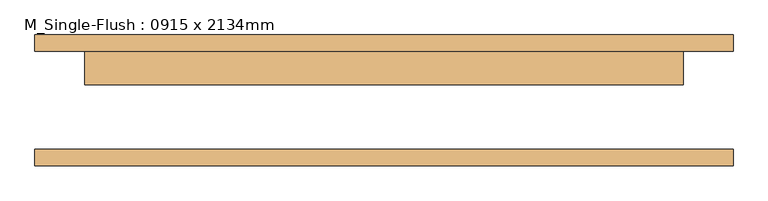
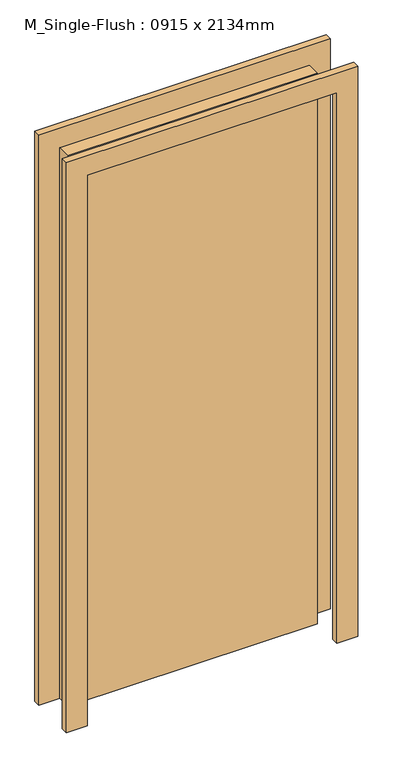
"""IFC4 building model written with IfcOpenShell, lengths in millimetres: door geometry, M_Single-Flush : 0915 x 2134mm."""

from ifc_helpers import new_model, si_unit, frame, origin, origin_with_axes, place, context, project, spatial, polyline, outline, extrude, source, transform, mapped, element, save


def m_single_flush_0915_x_2134mm_138fd904(model_context):
    return source(origin(), model_context, "Body", "SweptSolid", [
        extrude(outline(polyline([(2210.0, -533.5), (0.0, -533.5), (0.0, -457.5), (2134.0, -457.5), (2134.0, 457.5), (0.0, 457.5), (0.0, 533.5), (2210.0, 533.5), (2210.0, -533.5)])), frame((0.0, 75.0, 0.0), z_axis=(0.0, 1.0, 0.0), x_axis=(0.0, 0.0, 1.0)), (0.0, 0.0, 1.0), 25.0),
        extrude(outline(polyline([(2210.0, 533.5), (2210.0, -533.5), (0.0, -533.5), (0.0, -457.5), (2134.0, -457.5), (2134.0, 457.5), (0.0, 457.5), (0.0, 533.5), (2210.0, 533.5)])), frame((0.0, -100.0, 0.0), z_axis=(0.0, 1.0, 0.0), x_axis=(0.0, 0.0, 1.0)), (0.0, 0.0, 1.0), 25.0),
        extrude(outline(polyline([(457.5, 24.0), (-457.5, 24.0), (-457.5, 75.0), (457.5, 75.0), (457.5, 24.0)])), origin_with_axes(), (0.0, 0.0, 1.0), 2134.0),
    ])


if __name__ == "__main__":
    model = new_model("IFC4")
    model_context = context("Model", 3, world=origin())
    ifc_project = project(units=[si_unit("LENGTHUNIT", "METRE", prefix="MILLI")], contexts=[model_context])
    site = spatial("IfcSite", under=ifc_project)
    building = spatial("IfcBuilding", under=site)
    placement = place(None, origin())
    m_single_flush_0915_x_2134mm_shape = m_single_flush_0915_x_2134mm_138fd904(model_context)
    element("IfcDoor", 1, ObjectType="M_Single-Flush : 0915 x 2134mm", at=placement, inside=building, context=model_context, shape_type="MappedRepresentation", body=[
        mapped(m_single_flush_0915_x_2134mm_shape, transform((0.0, 0.0, 0.0), x_axis=(1.0, 0.0, 0.0), y_axis=(0.0, 1.0, 0.0), z_axis=(0.0, 0.0, 1.0))),
    ])
    save(model, "model.ifc")

# Revit data of these elements
# Type "M_Single-Flush : 0915 x 2134mm"
#   Type Mark = "20"
#   Construction Type Id = "MDOOR"
#   Analytic Construction = "Metal"
#   Thickness = 0.051 m
#   Thermal Resistance (R) = 0.270117 (m²·K)/W
#   Heat Transfer Coefficient (U) = 3.7021 W/(m²·K)
#   Height = 2.134 m
#   Trim Projection Ext = 0.025 m
#   Trim Projection Int = 0.025 m
#   Trim Width = 0.076 m
#   Width = 0.915 m
#   Define Thermal Properties by = 1
#   Define Thermal Properties by = 1
#   Door Material = Door - Panel
#   Frame Material = Door - Frame
#   Visual Light Transmittance = 0
#   Solar Heat Gain Coefficient = 0
#   Function = (empty or 0)
#   Wall Closure = (empty or 0)
# Element 1 (IfcDoor, "M_Single-Flush : 0915 x 2134mm")
#   Materials on its faces: "Door - Frame", "Door - Panel"
# Materials
#   "Door - Panel": class "Wood", colour RGB 210 159 95, transparency 0, Cost = 0
#   "Door - Frame": colour RGB 118 70 51, transparency 0, Cost = 0
